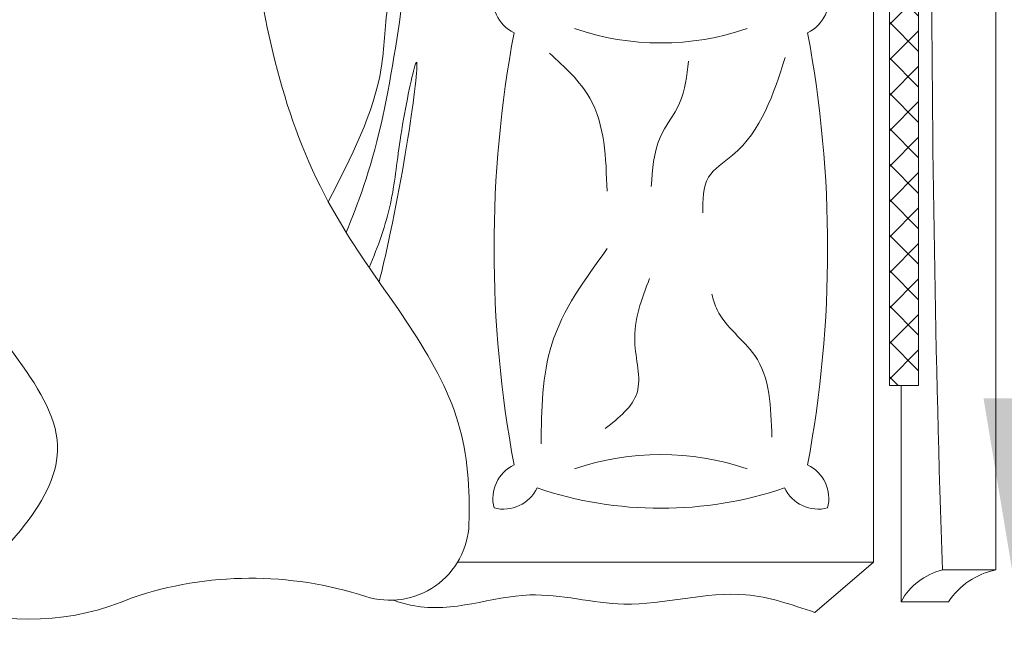
# Model space of a CAD drawing. Units: inches. Extents: x 2083 to 3317, y 1141 to 2115.
# Tile 239 of 256: x 3068 to 3114, y 1299 to 1327. Entities that reach past the tile are written whole.
import ezdxf

# ---------------------------------------------------------------- set-up
doc = ezdxf.new("R2010")
doc.units = ezdxf.units.IN
for name, color, linetype, lineweight in [('A-ANNO-DIMS', 2, 'Continuous', 18), ('A-FURN', 8, 'Continuous', 18), ('www.cadblocksfree.com', 7, 'Continuous', 9)]:
    doc.layers.add(name, color=color, linetype=linetype, lineweight=lineweight)
doc.layers.add('A-WALL-PATT', color=251, linetype='Continuous', lineweight=13, true_color=0x636466)
doc.styles.get("Standard").update_dxf_attribs({"font": 'arial.ttf'})
doc.dimstyles.new('ISO-25', dxfattribs={"dimtxt": 12, "dimasz": 12, "dimexe": 1.25, "dimexo": 0.625, "dimtad": 1, "dimlunit": 3, "dimtxsty": 'Standard', "dimcen": 2.5, "dimadec": 0, "dimazin": 0, "dimtfac": 1, "dimtmove": 0, "dimatfit": 3, "dimfxl": 1, "dimarcsym": 0})

# ---------------------------------------------------------------- blocks, each defined once
blk = doc.blocks.new('bed')
at = {"layer": 'www.cadblocksfree.com', "ltscale": 0.2}
h = blk.add_hatch(dxfattribs=at)
h.set_pattern_fill('ANSI37,_O', color=256, scale=0.393701)
h.set_pattern_definition([(45, (2420.7222, -262.9689), (-0.8838835, 0.8838835), []), (135, (2420.7222, -262.9689), (-0.8838835, -0.8838835), [])])
h.paths.add_polyline_path([(3417.573, 1472.402), (3372.192, 1472.402), (3372.192, 1470.941), (3417.573, 1470.941)])
for p, q in [((3426.763, 1473.586), (3426.763, 1476.249)), ((3372.192, 1472.402), (3417.573, 1472.402)), ((3417.573, 1470.941), (3417.573, 1472.402)), ((3372.192, 1470.941), (3417.573, 1470.941)), ((3426.379, 1470.154), (3428.883, 1467.22)), ((3409.943, 1443.853), (3408.408, 1442.961))]:
    blk.add_line(p, q, dxfattribs=at)
for points in [[(3426.763, 1476.249), (3363.002, 1476.249)], [(3417.573, 1471.524), (3428.347, 1471.524), (3428.347, 1473.886)], [(3426.379, 1449.413), (3426.379, 1470.154), (3363.387, 1470.154), (3363.387, 1447.076)]]:
    blk.add_lwpolyline(points, dxfattribs=at)
for centre, radius, start, end in [((3430.432, 1476.997), 3.744, 191.5225, 236.1729), ((3394.883, 2431.358), 958.303, 268.093559, 271.906441), ((3429.921, 1474.373), 3.255, 194.0061, 241.0824), ((3398.298, 1466.054), 1.87, 25.7901, 104.4834), ((3410.752, 1409.187), 58.677, 79.42346, 100.57654), ((3423.206, 1466.054), 1.87, 75.5166, 154.2099), ((3421.863, 1467.396), 1.87, 295.7901, 14.4834), ((3404.477, 1459.547), 19.215, 341.2852, 18.7148), ((3387.154, 1459.547), 13.338, 341.1598, 18.8402), ((3434.35, 1459.547), 13.338, 161.1598, 198.8402), ((3421.863, 1451.698), 1.87, 345.5166, 64.2099), ((3398.298, 1453.041), 1.87, 255.5166, 334.2099), ((3410.752, 1509.907), 58.677, 259.42346, 280.57654), ((3423.206, 1453.041), 1.87, 205.7901, 284.4834), ((3424.339, 1446.045), 3.937, 342.0511, 87.9851), ((3445.776, 1439.101), 18.596, 162.0511, 198.5657), ((3416.575, 1428.082), 12.646, 341.0268, 23.7782)]:
    blk.add_arc(centre, radius, start, end, dxfattribs=at)
for points, knots in [([(3428.883, 1467.22), (3428.494, 1466.08), (3427.438, 1462.983), (3429.036, 1458.154), (3427.377, 1452.621), (3429.083, 1448.872), (3428.374, 1446.522), (3428.273, 1446.192)], [0, 0, 0, 0, 0.0901802, 0.2449351, 0.3646438, 0.5132331, 0.5378548, 0.5378548, 0.5378548, 0.5378548]), ([(3401.221, 1465.744), (3403.047, 1465.161), (3405.408, 1464.407), (3407.088, 1461.635), (3408.312, 1461.638), (3408.953, 1461.64)], [0, 0, 0, 0, 5.530688, 7.154877, 8.940839, 8.940839, 8.940839, 8.940839]), ([(3420.141, 1465.083), (3418.661, 1465.041), (3416.141, 1464.969), (3414.502, 1462.52), (3413.283, 1462.165), (3413.011, 1462.086)], [0, 0, 0, 0, 4.163459, 7.093919, 7.934624, 7.934624, 7.934624, 7.934624]), ([(3401.408, 1460.927), (3402.126, 1460.846), (3403.512, 1460.689), (3405.283, 1459.224), (3406.806, 1459.127), (3407.654, 1459.073)], [0, 0, 0, 0, 2.127543, 4.10272, 6.58647, 6.58647, 6.58647, 6.58647]), ([(3419.716, 1456.774), (3419.174, 1457.459), (3418.052, 1458.876), (3415.084, 1457.893), (3413.26, 1458.594), (3412.241, 1458.985)], [0, 0, 0, 0, 2.388143, 4.935423, 8.166198, 8.166198, 8.166198, 8.166198]), ([(3400.996, 1453.995), (3401.698, 1454.761), (3403.498, 1456.726), (3406.222, 1456.811), (3407.884, 1456.863)], [0, 0, 0, 0, 3.013696, 7.735839, 7.735839, 7.735839, 7.735839]), ([(3420.479, 1453.579), (3418.77, 1453.599), (3415.179, 1453.639), (3412.269, 1455.762), (3410.745, 1456.874)], [0, 0, 0, 0, 5.002087, 10.507046, 10.507046, 10.507046, 10.507046]), ([(3409.943, 1443.853), (3413.12, 1445.837), (3417.433, 1449.66), (3422.724, 1450.042), (3424.477, 1449.98)], [1.3582378, 1.3582378, 1.3582378, 1.3582378, 1.6381418, 1.7706953, 1.7706953, 1.7706953, 1.7706953]), ([(3412.402, 1445.499), (3411.605, 1445.698), (3406.242, 1446.932), (3398.173, 1447.93), (3405.397, 1446.464), (3408.571, 1446.191), (3410.626, 1445.456), (3411.681, 1445)], [0.1043639, 0.1043639, 0.1043639, 0.1043639, 0.1489731, 0.3882761, 0.4793617, 0.5593494, 0.6446217, 0.6446217, 0.6446217, 0.6446217]), ([(3409.943, 1443.853), (3408.469, 1444.451), (3404.443, 1446.042), (3391.397, 1447.599), (3398.64, 1445.767), (3402.973, 1445.759), (3406.219, 1444.095), (3408.408, 1442.961)], [0.0056315, 0.0056315, 0.0056315, 0.0056315, 0.1489731, 0.3882761, 0.4793617, 0.5593494, 0.7397317, 0.7397317, 0.7397317, 0.7397317]), ([(3362.928, 1430.813), (3365.944, 1432.958), (3375.455, 1438.993), (3392.12, 1438.03), (3404.249, 1440.73), (3408.408, 1442.961)], [0.102872, 0.102872, 0.102872, 0.102872, 0.37972, 0.957702, 1.313793, 1.313793, 1.313793, 1.313793]), ([(3365.512, 1424.213), (3370.519, 1427.004), (3381.149, 1429.825), (3396.214, 1425.866), (3410.541, 1420.654), (3420.273, 1432.695), (3425.882, 1426.771), (3428.534, 1423.97)], [0.099185, 0.099185, 0.099185, 0.099185, 0.523647, 0.927087, 1.289918, 1.564439, 1.810555, 1.810555, 1.810555, 1.810555])]:
    blk.add_open_spline(points, degree=3, knots=knots, dxfattribs=at)
blk = doc.blocks.new('*D26')
at = {"layer": 'A-ANNO-DIMS', "color": 0, "lineweight": -2, "transparency": 16777216}
for p, q in [((3088.986, 1274.915), (3088.986, 1270.952)), ((3111.24, 1274.915), (3111.24, 1270.952)), ((3076.986, 1272.202), (2840.262, 1272.202)), ((3111.24, 1272.202), (3088.986, 1272.202)), ((3123.24, 1272.202), (3135.24, 1272.202))]:
    blk.add_line(p, q, dxfattribs=at)
at = {"layer": 'A-ANNO-DIMS', "color": 0, "transparency": 16777216}
for points in [[(3076.986, 1274.202), (3076.986, 1270.202), (3088.986, 1272.202)], [(3123.24, 1274.202), (3123.24, 1270.202), (3111.24, 1272.202)]]:
    blk.add_solid(points, dxfattribs=at)
at = {"layer": 'Defpoints', "color": 0, "transparency": 16777216}
for p in [(3088.986, 1275.54), (3111.24, 1275.54), (3088.986, 1272.202)]:
    blk.add_point(p, dxfattribs=at)
at = {"layer": 'A-ANNO-DIMS', "color": 0, "transparency": 16777216, "insert": (2952.624, 1279.032), "char_height": 12, "attachment_point": 5}
blk.add_mtext('NIGHTSTAND 1\'-10 1/2" TYP.', dxfattribs=at)
blk = doc.blocks.new('*D27')
at = {"layer": 'A-ANNO-DIMS', "color": 0, "lineweight": -2, "transparency": 16777216}
for p, q in [((3114.578, 1309.794), (3114.578, 1321.794)), ((3111.865, 1297.794), (3115.828, 1297.794)), ((3114.578, 1297.794), (3114.578, 1275.54)), ((3111.865, 1275.54), (3115.828, 1275.54)), ((3114.578, 1263.54), (3114.578, 1140.989))]:
    blk.add_line(p, q, dxfattribs=at)
at = {"layer": 'A-ANNO-DIMS', "color": 0, "transparency": 16777216}
for points in [[(3112.578, 1309.794), (3116.578, 1309.794), (3114.578, 1297.794)], [(3112.578, 1263.54), (3116.578, 1263.54), (3114.578, 1275.54)]]:
    blk.add_solid(points, dxfattribs=at)
at = {"layer": 'Defpoints', "color": 0, "transparency": 16777216}
for p in [(3111.24, 1297.794), (3111.24, 1275.54), (3114.578, 1275.54)]:
    blk.add_point(p, dxfattribs=at)
at = {"layer": 'A-ANNO-DIMS', "color": 0, "transparency": 16777216, "insert": (3107.749, 1196.264), "char_height": 12, "attachment_point": 5, "rotation": 90}
blk.add_mtext('1\'-10 1/2" TYP.', dxfattribs=at)

msp = doc.modelspace()

# ---------------------------------------------------------------- hatches: boundary and pattern name
at = {"layer": 'A-WALL-PATT'}
h = msp.add_hatch(color=256, dxfattribs=at)
h.dxf.hatch_style = 1
h.paths.add_polyline_path([(3126.96, 2020.761), (2748.96, 2020.761), (2604.96, 2020.761), (2226.96, 2020.761), (2226.96, 1702.761), (2466.96, 1702.761), (2466.96, 1582.761), (2418.96, 1582.761), (2418.96, 1477.761), (2226.96, 1477.761), (2226.96, 1263.261), (2544.96, 1263.261), (2544.96, 1411.761), (2604.96, 1411.761), (2685.96, 1411.761), (2685.96, 1420.761), (2604.96, 1420.761), (2604.96, 1573.761), (2604.96, 1702.761), (2604.96, 2011.761), (2748.96, 2011.761), (2748.96, 1702.761), (2862.96, 1702.761), (2862.96, 1621.761), (2871.96, 1621.761), (2871.96, 1702.761), (2883.96, 1702.761), (2883.96, 1706.939, -0.026459), (2883.96, 1711.761), (2757.96, 1711.761), (2757.96, 1807.761), (2787.96, 1807.761), (2787.96, 1812.261), (2757.96, 1812.261), (2757.96, 2011.761), (2877.96, 2011.761), (2877.96, 1812.261), (2847.96, 1812.261), (2847.96, 1807.761), (2889.836, 1807.761), (2889.836, 1812.261), (2882.46, 1812.261), (2882.46, 2011.761), (3117.96, 2011.761), (3117.96, 1812.261), (2937.836, 1812.261), (2937.836, 1807.761), (2995.71, 1807.761), (2995.71, 1796.118), (3000.21, 1796.118), (3000.21, 1807.761), (3117.96, 1807.761), (3117.96, 1711.761), (3000.21, 1711.761), (3000.21, 1760.118), (2998.573, 1760.118, -0.020711), (2995.71, 1760.118), (2995.71, 1711.761), (2931.96, 1711.761), (2931.96, 1702.761), (3126.96, 1702.761)])
h.paths.add_polyline_path([(2471.46, 2011.761), (2471.46, 1810.011), (2462.717, 1810.011), (2462.717, 1805.511), (2505.96, 1805.511), (2505.96, 1810.011), (2475.96, 1810.011), (2475.96, 2011.761), (2595.96, 2011.761), (2595.96, 1810.011), (2565.96, 1810.011), (2565.96, 1805.511), (2595.96, 1805.511), (2595.96, 1711.761), (2235.96, 1711.761), (2235.96, 1805.511), (2353.71, 1805.511), (2353.71, 1796.054), (2358.21, 1796.054), (2358.21, 1805.511), (2414.717, 1805.511), (2414.717, 1810.011), (2235.96, 1810.011), (2235.96, 2011.761)], flags=16)
h.paths.add_polyline_path([(2270.205, 1994.61), (2270.205, 1970.61), (2246.205, 1970.61), (2246.205, 1994.61)], flags=0)
edge = h.paths.add_edge_path(flags=0)
edge.add_ellipse((2332.027, 1899.798), major_axis=(-3.043, 3.043), ratio=0.168252, start_angle=-161.3322, end_angle=-156.3071, ccw=False)
edge.add_ellipse((2333.082, 1898.744), major_axis=(-1.055, 1.055), ratio=0.453532, start_angle=-123.371, end_angle=-94.1591)
edge = h.paths.add_edge_path(flags=0)
edge.add_ellipse((2332.027, 1968.876), major_axis=(3.043, 3.043), ratio=0.168252, start_angle=18.6678, end_angle=23.6929)
edge.add_spline(control_points=[(2332.926, 1970.691), (2332.227, 1970.336), (2330.894, 1969.659), (2328.413, 1970.932), (2327.204, 1967.749), (2324.71, 1969.956), (2322.533, 1967.012), (2320.013, 1971.296), (2317.68, 1968.158), (2316.041, 1967.102), (2315.427, 1966.81)], knot_values=[0, 0, 0, 0, 2.267059, 4.324559, 6.685584, 8.878641, 11.121502, 14.300359, 17.755284, 19.732645, 19.732645, 19.732645, 19.732645], degree=3, periodic=0)
edge.add_ellipse((2332.027, 1968.876), major_axis=(3.043, 3.043), ratio=0.168252, start_angle=18.6678, end_angle=23.6929, ccw=False)
edge.add_ellipse((2333.082, 1969.931), major_axis=(1.055, 1.055), ratio=0.453532, start_angle=56.629, end_angle=85.8409, ccw=False)
edge = h.paths.add_edge_path(flags=0)
edge.add_spline(control_points=[(2296.428, 1967.988), (2293.628, 1965.336), (2287.704, 1959.727), (2299.744, 1949.996), (2294.533, 1935.669), (2290.573, 1920.604), (2293.394, 1909.974), (2296.185, 1904.967)], knot_values=[0.099185, 0.099185, 0.099185, 0.099185, 0.345301, 0.619822, 0.982653, 1.386093, 1.810555, 1.810555, 1.810555, 1.810555], degree=3, periodic=0)
edge.add_spline(control_points=[(2296.185, 1904.967), (2297.384, 1902.619), (2298.001, 1901.949), (2298.553, 1901.468)], knot_values=[0.006246, 0.006246, 0.006246, 0.006246, 0.055476, 0.055476, 0.055476, 0.055476], degree=3, periodic=0)
edge.add_spline(control_points=[(2298.553, 1901.468), (2297.259, 1900.923), (2295.225, 1900.232), (2293.06, 1900.614), (2292.101, 1900.788), (2292.09, 1900.791)], knot_values=[0.312835, 0.312835, 0.312835, 0.312835, 0.40178, 0.474987, 0.475903, 0.475903, 0.475903, 0.475903], degree=3, periodic=0)
edge.add_arc((2292.794, 1904.664), 3.937, 215.4209, 259.6982, ccw=False)
edge.add_spline(control_points=[(2289.585, 1902.382), (2289.477, 1902.535), (2289.368, 1902.688), (2289.261, 1902.841)], knot_values=[0.102872, 0.102872, 0.102872, 0.102872, 0.116896, 0.116896, 0.116896, 0.116896], degree=3, periodic=0)
edge.add_spline(control_points=[(2289.261, 1902.841), (2288.687, 1902.55), (2287.64, 1902.02), (2285.881, 1901.874), (2283.853, 1901.504), (2281.72, 1899.711), (2278.467, 1899.493), (2276.157, 1901.883), (2272.259, 1899.804), (2267.778, 1901.843), (2262.244, 1900.184), (2257.415, 1901.782), (2254.318, 1900.726), (2253.178, 1900.337)], knot_values=[0, 0, 0, 0, 1.907977, 3.477176, 5.261074, 7.972851, 11.680248, 13.717921, 16.939592, 22.789562, 27.502503, 33.595215, 37.145618, 37.145618, 37.145618, 37.145618], degree=3, periodic=0)
edge.add_line((2253.178, 1900.337), (2250.244, 1902.841))
edge.add_line((2250.244, 1902.841), (2250.244, 1965.833))
edge.add_line((2250.244, 1965.833), (2253.178, 1968.337))
edge.add_spline(control_points=[(2253.178, 1968.337), (2254.318, 1967.948), (2257.415, 1966.892), (2262.244, 1968.49), (2267.778, 1966.831), (2271.527, 1968.537), (2273.876, 1967.828), (2274.207, 1967.728)], knot_values=[0, 0, 0, 0, 0.09018, 0.244935, 0.364644, 0.513233, 0.537855, 0.537855, 0.537855, 0.537855], degree=3, periodic=0)
edge.add_arc((2274.353, 1963.793), 3.937, 72.0511, 92.1279, ccw=False)
edge.add_arc((2281.297, 1985.23), 18.596, 252.0511, 288.5657)
edge.add_arc((2292.317, 1956.029), 12.646, 71.0268, 113.7782, ccw=False)
edge = h.paths.add_edge_path(flags=0)
edge.add_spline(control_points=[(2274.899, 1951.856), (2275.066, 1951.617), (2275.233, 1951.377), (2275.398, 1951.136)], knot_values=[1.409916, 1.409916, 1.409916, 1.409916, 1.43159, 1.43159, 1.43159, 1.43159], degree=3, periodic=0)
edge.add_spline(control_points=[(2275.398, 1951.136), (2275.792, 1950.562), (2276.179, 1949.984), (2276.546, 1949.397)], knot_values=[1.358238, 1.358238, 1.358238, 1.358238, 1.409916, 1.409916, 1.409916, 1.409916], degree=3, periodic=0)
edge.add_line((2276.546, 1949.397), (2277.437, 1947.862))
edge.add_spline(control_points=[(2277.437, 1947.862), (2276.304, 1945.673), (2274.64, 1942.427), (2274.632, 1938.094), (2272.799, 1930.852), (2274.356, 1943.897), (2275.948, 1947.923), (2276.546, 1949.397)], knot_values=[0.005632, 0.005632, 0.005632, 0.005632, 0.186014, 0.266002, 0.357087, 0.59639, 0.739732, 0.739732, 0.739732, 0.739732], degree=3, periodic=0)
edge.add_spline(control_points=[(2276.546, 1949.397), (2276.179, 1949.984), (2275.792, 1950.562), (2275.398, 1951.136)], knot_values=[1.358238, 1.358238, 1.358238, 1.358238, 1.409916, 1.409916, 1.409916, 1.409916], degree=3, periodic=0)
edge.add_spline(control_points=[(2275.398, 1951.136), (2274.943, 1950.08), (2274.208, 1948.025), (2273.935, 1944.851), (2272.469, 1937.627), (2273.466, 1945.696), (2274.701, 1951.059), (2274.899, 1951.856)], knot_values=[0.104364, 0.104364, 0.104364, 0.104364, 0.189636, 0.269624, 0.36071, 0.600013, 0.644622, 0.644622, 0.644622, 0.644622], degree=3, periodic=0)
h.paths.add_polyline_path([(2269.168, 1963.128, -0.357527), (2268.171, 1960.976, -0.092561), (2268.171, 1939.436, -0.357527), (2269.168, 1937.285, -0.357527), (2267.016, 1938.282, -0.164785), (2254.686, 1938.282, -0.357527), (2252.534, 1937.285, -0.357527), (2253.531, 1939.436, -0.092561), (2253.531, 1960.976, -0.357527), (2252.534, 1963.128, -0.357527), (2254.686, 1962.131, -0.164785), (2267.016, 1962.131, -0.357527)], flags=0)
h.paths.add_polyline_path([(2248.874, 1967.802), (2248.874, 1957.028), (2249.458, 1957.028), (2249.458, 1911.647), (2248.874, 1911.647), (2248.874, 1900.873), (2246.512, 1900.873, 0.197327), (2244.15, 1902.457), (2244.15, 1966.218, 0.197327), (2246.512, 1967.802)], flags=0)
h.paths.add_polyline_path([(2269.168, 1931.389, -0.357527), (2268.171, 1929.238, -0.092561), (2268.171, 1907.698, -0.357527), (2269.168, 1905.547, -0.357527), (2267.016, 1906.544, -0.164785), (2254.686, 1906.544, -0.357527), (2252.534, 1905.547, -0.357527), (2253.531, 1907.698, -0.092561), (2253.531, 1929.238, -0.357527), (2252.534, 1931.389, -0.357527), (2254.686, 1930.392, -0.164785), (2267.016, 1930.392, -0.357527)], flags=0)
edge = h.paths.add_edge_path(flags=0)
edge.add_spline(control_points=[(2276.197, 1906.724), (2276.168, 1909.029), (2276.114, 1913.372), (2270.598, 1924.925), (2273.905, 1919.013), (2275.922, 1916.262), (2275.475, 1912.402), (2277.258, 1910.381), (2276.696, 1908.225), (2276.646, 1906.813), (2276.618, 1906.008)], knot_values=[0, 0, 0, 0, 8.61026, 16.221274, 18.843057, 23.804898, 27.440828, 29.356102, 31.203478, 33.650687, 33.650687, 33.650687, 33.650687], degree=3, periodic=0)
edge.add_spline(control_points=[(2276.618, 1906.008), (2276.623, 1905.624), (2276.498, 1904.629), (2275.442, 1903.855), (2274.937, 1903.08), (2274.859, 1902.841)], knot_values=[0.156488, 0.156488, 0.156488, 0.156488, 0.184398, 0.231376, 0.250598, 0.250598, 0.250598, 0.250598], degree=3, periodic=0)
edge.add_line((2274.859, 1902.841), (2276.506, 1902.841))
edge.add_spline(control_points=[(2276.506, 1902.841), (2276.788, 1903.085), (2277.665, 1904.125), (2278.25, 1904.341), (2277.654, 1908.527), (2278.156, 1906.228), (2278.1, 1905.286), (2278.847, 1904.069), (2277.857, 1903.415), (2277.874, 1902.991), (2277.904, 1902.841)], knot_values=[0.059574, 0.059574, 0.059574, 0.059574, 0.080753, 0.103741, 0.16972, 0.176036, 0.207137, 0.240474, 0.262341, 0.27366, 0.27366, 0.27366, 0.27366], degree=3, periodic=0)
edge.add_line((2277.904, 1902.841), (2280.03, 1902.841))
edge.add_spline(control_points=[(2280.03, 1902.841), (2279.888, 1903.088), (2279.499, 1903.982), (2280.152, 1905.939), (2278.104, 1909.658), (2279.762, 1907.185), (2280.328, 1904.875), (2280.485, 1903.49), (2281.463, 1903.249), (2281.758, 1902.936), (2281.834, 1902.841)], knot_values=[0.013856, 0.013856, 0.013856, 0.013856, 0.034874, 0.088867, 0.107879, 0.126738, 0.158714, 0.193757, 0.217487, 0.226722, 0.226722, 0.226722, 0.226722], degree=3, periodic=0)
edge.add_spline(control_points=[(2281.834, 1902.841), (2281.788, 1902.827), (2281.647, 1902.783), (2281.396, 1902.859), (2281.088, 1902.985), (2280.721, 1903.061), (2280.333, 1903.026), (2280.125, 1902.899), (2280.03, 1902.841)], knot_values=[0, 0, 0, 0, 0.14413, 0.435517, 0.749276, 1.153046, 1.548371, 1.878348, 1.878348, 1.878348, 1.878348], degree=3, periodic=0)
edge.add_line((2280.03, 1902.841), (2277.904, 1902.841))
edge.add_spline(control_points=[(2277.904, 1902.841), (2277.893, 1902.796), (2277.865, 1902.68), (2277.607, 1902.687), (2277.274, 1902.801), (2276.838, 1902.62), (2276.584, 1902.789), (2276.506, 1902.841)], knot_values=[0, 0, 0, 0, 0.127189, 0.326199, 0.628009, 1.24357, 1.515331, 1.515331, 1.515331, 1.515331], degree=3, periodic=0)
edge.add_line((2276.506, 1902.841), (2274.859, 1902.841))
edge.add_spline(control_points=[(2274.859, 1902.841), (2274.814, 1902.899), (2274.725, 1903.013), (2274.493, 1903.119), (2274.244, 1902.961), (2273.937, 1903.185), (2273.614, 1902.983), (2273.408, 1902.883), (2273.322, 1902.841)], knot_values=[0, 0, 0, 0, 0.21843, 0.436957, 0.687977, 0.990379, 1.398396, 1.69185, 1.69185, 1.69185, 1.69185], degree=3, periodic=0)
edge.add_spline(control_points=[(2273.322, 1902.841), (2273.617, 1903.446), (2274.274, 1904.538), (2276.027, 1904.574), (2276.207, 1906.584), (2276.197, 1906.724)], knot_values=[0.012227, 0.012227, 0.012227, 0.012227, 0.059472, 0.106218, 0.134458, 0.134458, 0.134458, 0.134458], degree=3, periodic=0)
h.paths.add_polyline_path([(2270.776, 1897.79), (2270.776, 1873.79), (2246.776, 1873.79), (2246.776, 1897.79)], flags=0)
h.paths.add_polyline_path([(2353.71, 1760.005), (2353.71, 1760.054), (2358.21, 1760.054, -0.033729)], flags=0)
h.paths.add_polyline_path([(2321.819, 1737.529), (2341.995, 1737.529, -0.414214), (2343.203, 1736.321), (2343.203, 1721.021, -0.414214), (2341.995, 1719.813), (2321.819, 1719.813, -0.414214), (2320.611, 1721.021), (2320.611, 1736.321, -0.414214)], flags=0)
h.paths.add_polyline_path([(2324.235, 1736.321), (2339.579, 1736.321, -0.414214), (2341.995, 1733.905), (2341.995, 1725.45, -0.414214), (2339.579, 1723.034), (2333.681, 1723.034), (2333.845, 1722.045, -0.870646), (2335.425, 1721.826, -0.767327), (2333.923, 1721.423), (2331.291, 1721.423, -0.767327), (2329.788, 1721.826, -0.870646), (2331.368, 1722.045), (2331.533, 1723.034), (2324.235, 1723.034, -0.414214), (2321.819, 1725.45), (2321.819, 1733.905, -0.414214)], flags=0)
h.paths.add_polyline_path([(2570.484, 1928.615), (2589.684, 1928.615), (2590.169, 1928.615), (2590.169, 1904.993), (2570.484, 1904.993)], flags=0)
h.paths.add_polyline_path([(2574.447, 1927.264, -1), (2572.829, 1927.264, -1)], flags=0)
h.paths.add_polyline_path([(2573.09, 1926.941), (2573.925, 1927.776), (2574.148, 1927.553), (2573.313, 1926.718)], flags=0)
h.paths.add_polyline_path([(2578.779, 1919.73, -1), (2571.592, 1919.73, -1)], flags=0)
h.paths.add_polyline_path([(2578.385, 1919.73, -1), (2571.985, 1919.73, -1)], flags=0)
h.paths.add_polyline_path([(2331.596, 1729.476, -1), (2333.618, 1729.476, -1)], flags=0)
h.paths.add_polyline_path([(2578.034, 1927.264, -1), (2576.416, 1927.264, -1)], flags=0)
h.paths.add_polyline_path([(2576.689, 1927.531), (2576.912, 1927.754), (2577.747, 1926.919), (2577.524, 1926.696)], flags=0)
h.paths.add_polyline_path([(2578.139, 1909.86, -1), (2572.232, 1909.86, -1)], flags=0)
h.paths.add_polyline_path([(2577.745, 1909.86, -1), (2572.625, 1909.86, -1)], flags=0)
h.paths.add_polyline_path([(2583.798, 1927.264, -1), (2582.179, 1927.264, -1)], flags=0)
h.paths.add_polyline_path([(2582.719, 1927.754), (2583.554, 1926.919), (2583.331, 1926.696), (2582.496, 1927.531)], flags=0)
h.paths.add_polyline_path([(2582.496, 1927.531), (2582.719, 1927.754), (2583.554, 1926.919), (2583.331, 1926.696)], flags=0)
h.paths.add_polyline_path([(2587.739, 1920.53, -1), (2581.832, 1920.53, -1)], flags=0)
h.paths.add_polyline_path([(2587.345, 1920.53, -1), (2582.225, 1920.53, -1)], flags=0)
h.paths.add_polyline_path([(2587.385, 1927.264, -1), (2585.766, 1927.264, -1)], flags=0)
h.paths.add_polyline_path([(2586.082, 1926.98), (2586.917, 1927.815), (2587.14, 1927.593), (2586.305, 1926.758)], flags=0)
h.paths.add_polyline_path([(2588.379, 1910.66, -1), (2581.192, 1910.66, -1)], flags=0)
h.paths.add_polyline_path([(2587.985, 1910.66, -1), (2581.585, 1910.66, -1)], flags=0)
h.paths.add_polyline_path([(2417.168, 1729.478), (2437.344, 1729.478, -0.414214), (2438.552, 1728.27), (2438.552, 1712.969, -0.414214), (2437.344, 1711.761), (2417.168, 1711.761, -0.414214), (2415.96, 1712.969), (2415.96, 1728.27, -0.414214)], flags=0)
h.paths.add_polyline_path([(2419.584, 1728.27), (2434.928, 1728.27, -0.414214), (2437.344, 1725.854), (2437.344, 1717.398, -0.414214), (2434.928, 1714.983), (2429.029, 1714.983), (2429.194, 1713.994, -0.870646), (2430.774, 1713.775, -0.767327), (2429.271, 1713.372), (2426.64, 1713.372, -0.767327), (2425.137, 1713.775, -0.870646), (2426.717, 1713.994), (2426.882, 1714.983), (2419.584, 1714.983, -0.414214), (2417.168, 1717.398), (2417.168, 1725.854, -0.414214)], flags=0)
h.paths.add_polyline_path([(2419.584, 1728.27), (2434.928, 1728.27, -0.414214), (2437.344, 1725.854), (2437.344, 1717.398, -0.414214), (2434.928, 1714.983), (2429.029, 1714.983), (2428.358, 1719.009), (2427.553, 1719.009), (2426.882, 1714.983), (2419.584, 1714.983, -0.414214), (2417.168, 1717.398), (2417.168, 1725.854, -0.414214)], flags=0)
h.paths.add_polyline_path([(2426.944, 1721.425, -1), (2428.967, 1721.425, -1)], flags=0)
h.paths.add_polyline_path([(2475.96, 1702.761), (2595.96, 1702.761), (2595.96, 1582.761), (2475.96, 1582.761)], flags=16)
h.paths.add_polyline_path([(2427.96, 1573.761), (2595.96, 1573.761), (2595.96, 1468.761), (2595.96, 1420.761), (2384.46, 1420.761), (2384.46, 1468.761), (2427.96, 1468.761)], flags=16)
h.paths.add_polyline_path([(2379.96, 1468.761), (2379.96, 1420.761), (2235.96, 1420.761), (2235.96, 1468.761)], flags=16)
h.paths.add_polyline_path([(2317.816, 1466.696), (2337.992, 1466.696, -0.414214), (2339.2, 1465.488), (2339.2, 1450.187, -0.414214), (2337.992, 1448.979), (2317.816, 1448.979, -0.414214), (2316.608, 1450.187), (2316.608, 1465.488, -0.414214)], flags=0)
h.paths.add_polyline_path([(2320.232, 1465.488), (2335.576, 1465.488, -0.414214), (2337.992, 1463.072), (2337.992, 1454.616, -0.414214), (2335.576, 1452.2), (2329.677, 1452.2), (2329.842, 1451.212, -0.870646), (2331.422, 1450.992, -0.767327), (2329.92, 1450.59), (2327.288, 1450.59, -0.767327), (2325.785, 1450.992, -0.870646), (2327.365, 1451.212), (2327.53, 1452.2), (2320.232, 1452.2, -0.414214), (2317.816, 1454.616), (2317.816, 1463.072, -0.414214)], flags=0)
h.paths.add_polyline_path([(2320.232, 1465.488), (2335.576, 1465.488, -0.414214), (2337.992, 1463.072), (2337.992, 1454.616, -0.414214), (2335.576, 1452.2), (2329.677, 1452.2), (2329.006, 1456.227), (2328.201, 1456.227), (2327.53, 1452.2), (2320.232, 1452.2, -0.414214), (2317.816, 1454.616), (2317.816, 1463.072, -0.414214)], flags=0)
h.paths.add_polyline_path([(2327.593, 1458.643, -1), (2329.615, 1458.643, -1)], flags=0)
h.paths.add_polyline_path([(2244.412, 1433.34), (2241.921, 1433.34, -0.414214), (2240.018, 1435.244), (2240.018, 1440.953, -0.414211), (2241.921, 1442.856), (2244.412, 1442.856, -1.976472)], flags=0)
h.paths.add_polyline_path([(2245.357, 1434.398, -0.414214), (2245.357, 1441.799, -2.144098)], flags=0)
h.paths.add_polyline_path([(2535.96, 1416.261), (2535.96, 1272.261), (2235.96, 1272.261), (2235.96, 1416.261)], flags=16)
h.paths.add_polyline_path([(2260.12, 1384.293), (2260.12, 1362.039), (2237.865, 1362.039), (2237.865, 1384.293)], flags=0)
edge = h.paths.add_edge_path(flags=0)
edge.add_line((2318.252, 1362.093), (2318.146, 1362.001))
edge.add_ellipse((2317.445, 1360.431), major_axis=(2.822, 2.822), ratio=0.168252, start_angle=18.6678, end_angle=20.9481, ccw=False)
edge.add_ellipse((2318.423, 1361.409), major_axis=(0.978, 0.978), ratio=0.453532, start_angle=56.629, end_angle=70.2262, ccw=False)
edge = h.paths.add_edge_path(flags=0)
edge.add_line((2319.107, 1295.571), (2319.015, 1295.677))
edge.add_ellipse((2317.445, 1296.378), major_axis=(-2.822, 2.822), ratio=0.168252, start_angle=-161.3322, end_angle=-159.0519, ccw=False)
edge.add_ellipse((2318.423, 1295.4), major_axis=(-0.978, 0.978), ratio=0.453532, start_angle=-123.371, end_angle=-109.7738)
edge = h.paths.add_edge_path(flags=0)
edge.add_spline(control_points=[(2284.21, 1301.17), (2284.581, 1300.445), (2284.891, 1299.892), (2285.16, 1299.461)], knot_values=[0.039066, 0.039066, 0.039066, 0.039066, 0.055476, 0.055476, 0.055476, 0.055476], degree=3, periodic=0)
edge.add_line((2285.16, 1299.461), (2284.21, 1301.17))
edge = h.paths.add_edge_path(flags=0)
edge.add_line((2280.412, 1297.298), (2283.37, 1297.036))
edge.add_line((2283.37, 1297.036), (2286.406, 1297.926))
edge.add_spline(control_points=[(2286.406, 1297.926), (2285.305, 1297.463), (2284.345, 1297.129), (2283.37, 1297.036)], knot_values=[0.394369, 0.394369, 0.394369, 0.394369, 0.475903, 0.475903, 0.475903, 0.475903], degree=3, periodic=0)
edge.add_spline(control_points=[(2283.37, 1297.036), (2283.281, 1297.028), (2282.316, 1296.957), (2281.313, 1297.134), (2280.423, 1297.296), (2280.412, 1297.298)], knot_values=[0.312835, 0.312835, 0.312835, 0.312835, 0.320246, 0.393453, 0.394369, 0.394369, 0.394369, 0.394369], degree=3, periodic=0)
edge = h.paths.add_edge_path(flags=0)
edge.add_line((2284.436, 1359.607), (2280.446, 1355.328))
edge.add_line((2280.446, 1355.328), (2279.58, 1351.018))
edge.add_line((2279.58, 1351.018), (2282.413, 1346.58))
edge.add_spline(control_points=[(2282.413, 1346.58), (2283.153, 1345.589), (2284.253, 1344.029), (2284.801, 1342.387), (2284.935, 1341.806)], knot_values=[1.240098, 1.240098, 1.240098, 1.240098, 1.332892, 1.382712, 1.382712, 1.382712, 1.382712], degree=3, periodic=0)
edge.add_spline(control_points=[(2284.935, 1341.806), (2285.319, 1340.141), (2285.233, 1338.409), (2284.91, 1336.654)], knot_values=[1.097484, 1.097484, 1.097484, 1.097484, 1.240098, 1.240098, 1.240098, 1.240098], degree=3, periodic=0)
edge.add_spline(control_points=[(2284.91, 1336.654), (2284.587, 1334.899), (2284.027, 1333.12), (2283.463, 1331.361)], knot_values=[0.95487, 0.95487, 0.95487, 0.95487, 1.097484, 1.097484, 1.097484, 1.097484], degree=3, periodic=0)
edge.add_line((2283.463, 1331.361), (2281.89, 1326.153))
edge.add_line((2281.89, 1326.153), (2280.756, 1321.056))
edge.add_line((2280.756, 1321.056), (2280.299, 1316.002))
edge.add_line((2280.299, 1316.002), (2280.716, 1310.95))
edge.add_line((2280.716, 1310.95), (2282.028, 1305.972))
edge.add_line((2282.028, 1305.972), (2284.21, 1301.17))
edge.add_spline(control_points=[(2284.21, 1301.17), (2283.341, 1302.73), (2282.612, 1304.336), (2282.028, 1305.972)], knot_values=[0.099185, 0.099185, 0.099185, 0.099185, 0.241799, 0.241799, 0.241799, 0.241799], degree=3, periodic=0)
edge.add_spline(control_points=[(2282.028, 1305.972), (2281.444, 1307.608), (2281.005, 1309.273), (2280.716, 1310.95)], knot_values=[0.241799, 0.241799, 0.241799, 0.241799, 0.384413, 0.384413, 0.384413, 0.384413], degree=3, periodic=0)
edge.add_spline(control_points=[(2280.716, 1310.95), (2280.433, 1312.588), (2280.289, 1314.277), (2280.299, 1315.962), (2280.299, 1316.002)], knot_values=[0.384413, 0.384413, 0.384413, 0.384413, 0.523647, 0.527028, 0.527028, 0.527028, 0.527028], degree=3, periodic=0)
edge.add_spline(control_points=[(2280.299, 1316.002), (2280.312, 1317.687), (2280.478, 1319.368), (2280.756, 1321.056)], knot_values=[0.527028, 0.527028, 0.527028, 0.527028, 0.669642, 0.669642, 0.669642, 0.669642], degree=3, periodic=0)
edge.add_spline(control_points=[(2280.756, 1321.056), (2281.035, 1322.744), (2281.426, 1324.44), (2281.89, 1326.153)], knot_values=[0.669642, 0.669642, 0.669642, 0.669642, 0.812256, 0.812256, 0.812256, 0.812256], degree=3, periodic=0)
edge.add_spline(control_points=[(2281.89, 1326.153), (2282.264, 1327.533), (2282.788, 1329.262), (2283.353, 1331.018), (2283.463, 1331.361)], knot_values=[0.812256, 0.812256, 0.812256, 0.812256, 0.927087, 0.95487, 0.95487, 0.95487, 0.95487], degree=3, periodic=0)
edge.add_line((2283.463, 1331.361), (2284.91, 1336.654))
edge.add_line((2284.91, 1336.654), (2284.935, 1341.806))
edge.add_line((2284.935, 1341.806), (2282.413, 1346.58))
edge.add_spline(control_points=[(2282.413, 1346.58), (2281.275, 1348.104), (2280.078, 1349.57), (2279.58, 1351.018)], knot_values=[1.382712, 1.382712, 1.382712, 1.382712, 1.525326, 1.525326, 1.525326, 1.525326], degree=3, periodic=0)
edge.add_spline(control_points=[(2279.58, 1351.018), (2279.443, 1351.415), (2279.136, 1352.857), (2279.735, 1354.29), (2280.446, 1355.328)], knot_values=[1.525326, 1.525326, 1.525326, 1.525326, 1.564439, 1.667941, 1.667941, 1.667941, 1.667941], degree=3, periodic=0)
edge.add_spline(control_points=[(2280.446, 1355.328), (2281.426, 1356.758), (2282.931, 1358.183), (2284.436, 1359.607)], knot_values=[1.667941, 1.667941, 1.667941, 1.667941, 1.810555, 1.810555, 1.810555, 1.810555], degree=3, periodic=0)
edge.add_arc((2280.623, 1348.518), 11.726, 71.0268, 113.7782)
edge.add_arc((2270.405, 1375.595), 17.244, 252.0511, 288.5657, ccw=False)
edge.add_arc((2263.966, 1355.718), 3.651, 72.0511, 92.1279)
edge.add_arc((2263.966, 1355.718), 3.651, 92.1279, 177.9851)
edge.add_spline(control_points=[(2260.318, 1355.846), (2260.26, 1354.221), (2260.551, 1350.187), (2262.999, 1346.766), (2264.473, 1344.649)], knot_values=[1.43159, 1.43159, 1.43159, 1.43159, 1.564144, 1.770695, 1.770695, 1.770695, 1.770695], degree=3, periodic=0)
edge.add_line((2264.473, 1344.649), (2264.936, 1343.983))
edge.add_spline(control_points=[(2263.801, 1340.248), (2263.843, 1340.514), (2264.067, 1341.756), (2264.513, 1343.002), (2264.935, 1343.981)], knot_values=[0.53657, 0.53657, 0.53657, 0.53657, 0.559349, 0.644622, 0.644622, 0.644622, 0.644622], degree=3, periodic=0)
edge.add_spline(control_points=[(2264.935, 1343.981), (2265.118, 1343.715), (2265.299, 1343.448), (2265.477, 1343.179)], knot_values=[1.384077, 1.384077, 1.384077, 1.384077, 1.409916, 1.409916, 1.409916, 1.409916], degree=3, periodic=0)
edge.add_spline(control_points=[(2265.477, 1343.179), (2265.655, 1342.911), (2265.829, 1342.641), (2265.999, 1342.369)], knot_values=[1.358238, 1.358238, 1.358238, 1.358238, 1.384077, 1.384077, 1.384077, 1.384077], degree=3, periodic=0)
edge.add_line((2265.999, 1342.369), (2266.826, 1340.946))
edge.add_spline(control_points=[(2266.826, 1340.946), (2268.894, 1337.09), (2271.398, 1325.843), (2270.516, 1310.569), (2275.919, 1301.861), (2277.79, 1299.199)], knot_values=[0.116896, 0.116896, 0.116896, 0.116896, 0.472987, 1.050969, 1.313793, 1.313793, 1.313793, 1.313793], degree=3, periodic=0)
edge.add_spline(control_points=[(2277.79, 1299.199), (2277.839, 1299.128), (2277.889, 1299.057), (2277.94, 1298.987)], knot_values=[0.109884, 0.109884, 0.109884, 0.109884, 0.116896, 0.116896, 0.116896, 0.116896], degree=3, periodic=0)
edge.add_line((2277.94, 1298.987), (2277.789, 1299.199))
edge.add_spline(control_points=[(2277.789, 1299.199), (2277.257, 1298.929), (2276.286, 1298.438), (2275.039, 1298.334), (2274.383, 1298.239), (2274.215, 1298.209)], knot_values=[33.12187, 33.12187, 33.12187, 33.12187, 35.029056, 36.598255, 37.144827, 37.144827, 37.144827, 37.144827], degree=3, periodic=0)
edge.add_line((2274.215, 1298.209), (2273.073, 1297.893))
edge.add_spline(control_points=[(2273.073, 1297.893), (2272.323, 1297.58), (2271.039, 1296.511), (2269.248, 1296.226), (2268.423, 1296.375)], knot_values=[26.532584, 26.532584, 26.532584, 26.532584, 29.198919, 31.839101, 31.839101, 31.839101, 31.839101], degree=3, periodic=0)
edge.add_line((2268.423, 1296.375), (2263.879, 1297.458))
edge.add_spline(control_points=[(2263.879, 1297.458), (2263.556, 1297.359), (2261.86, 1296.839), (2260.239, 1297.282), (2258.933, 1297.516)], knot_values=[15.919551, 15.919551, 15.919551, 15.919551, 16.939592, 21.226067, 21.226067, 21.226067, 21.226067], degree=3, periodic=0)
edge.add_line((2258.933, 1297.516), (2254.055, 1297.329))
edge.add_spline(control_points=[(2254.055, 1297.329), (2253.756, 1297.296), (2252.114, 1297.165), (2250.462, 1297.544), (2249.13, 1297.668)], knot_values=[5.306517, 5.306517, 5.306517, 5.306517, 6.276435, 10.613034, 10.613034, 10.613034, 10.613034], degree=3, periodic=0)
edge.add_line((2249.13, 1297.668), (2244.332, 1296.878))
edge.add_line((2244.332, 1296.878), (2241.611, 1299.199))
edge.add_line((2241.611, 1299.199), (2241.611, 1357.609))
edge.add_line((2241.611, 1357.609), (2244.332, 1359.931))
edge.add_line((2244.332, 1359.931), (2252.729, 1359.543))
edge.add_spline(control_points=[(2252.729, 1359.543), (2252.871, 1359.546), (2253.306, 1359.548), (2253.74, 1359.514), (2254.032, 1359.482)], knot_values=[0.233291, 0.233291, 0.233291, 0.233291, 0.244935, 0.268927, 0.268927, 0.268927, 0.268927], degree=3, periodic=0)
edge.add_line((2254.032, 1359.482), (2259.587, 1359.416))
edge.add_spline(control_points=[(2259.587, 1359.416), (2260.677, 1359.629), (2262.073, 1359.897), (2263.524, 1359.459), (2263.83, 1359.366)], knot_values=[0.422516, 0.422516, 0.422516, 0.422516, 0.513233, 0.537855, 0.537855, 0.537855, 0.537855], degree=3, periodic=0)
edge.add_arc((2263.966, 1355.718), 3.651, 72.0511, 92.1279, ccw=False)
edge.add_arc((2270.405, 1375.595), 17.244, 252.0511, 288.5657)
edge.add_arc((2280.623, 1348.518), 11.726, 71.0268, 113.7782, ccw=False)
h.paths.add_polyline_path([(2240.341, 1359.435), (2240.341, 1349.444), (2240.882, 1349.444), (2240.882, 1307.365), (2240.341, 1307.365), (2240.341, 1297.374), (2238.15, 1297.374, 0.197327), (2235.96, 1298.843), (2235.96, 1357.966, 0.197327), (2238.15, 1359.435)], flags=0)
h.paths.add_polyline_path([(2259.158, 1355.101, -0.357527), (2258.233, 1353.106, -0.092561), (2258.233, 1333.133, -0.357527), (2259.158, 1331.138, -0.357527), (2257.163, 1332.062, -0.164785), (2245.729, 1332.062, -0.357527), (2243.735, 1331.138, -0.357527), (2244.659, 1333.133, -0.092561), (2244.659, 1353.106, -0.357527), (2243.735, 1355.101, -0.357527), (2245.729, 1354.176, -0.164785), (2257.163, 1354.176, -0.357527)], flags=0)
edge = h.paths.add_edge_path(flags=0)
edge.add_line((2265.999, 1342.369), (2266.826, 1340.946))
edge.add_line((2266.826, 1340.946), (2265.308, 1337.814))
edge.add_line((2265.308, 1337.814), (2264.358, 1334.653))
edge.add_line((2264.358, 1334.653), (2264.262, 1333.8))
edge.add_spline(control_points=[(2264.262, 1333.8), (2264.208, 1333.187), (2264.162, 1332.366), (2264.007, 1331.414), (2263.969, 1331.202)], knot_values=[0.464444, 0.464444, 0.464444, 0.464444, 0.516691, 0.531608, 0.531608, 0.531608, 0.531608], degree=3, periodic=0)
edge.add_spline(control_points=[(2263.969, 1331.202), (2263.775, 1330.119), (2263.424, 1328.791), (2263.257, 1328.531), (2263.234, 1328.515)], knot_values=[0.372682, 0.372682, 0.372682, 0.372682, 0.44885, 0.464444, 0.464444, 0.464444, 0.464444], degree=3, periodic=0)
edge.add_spline(control_points=[(2263.234, 1328.515), (2263.096, 1328.42), (2263.131, 1329.301), (2263.275, 1330.616)], knot_values=[0.280919, 0.280919, 0.280919, 0.280919, 0.372682, 0.372682, 0.372682, 0.372682], degree=3, periodic=0)
edge.add_spline(control_points=[(2263.275, 1330.616), (2263.419, 1331.93), (2263.672, 1333.677), (2263.97, 1335.315)], knot_values=[0.189157, 0.189157, 0.189157, 0.189157, 0.280919, 0.280919, 0.280919, 0.280919], degree=3, periodic=0)
edge.add_spline(control_points=[(2263.97, 1335.315), (2264.1, 1336.032), (2264.419, 1337.622), (2264.755, 1338.864), (2264.947, 1339.491)], knot_values=[0.097394, 0.097394, 0.097394, 0.097394, 0.137578, 0.189157, 0.189157, 0.189157, 0.189157], degree=3, periodic=0)
edge.add_spline(control_points=[(2264.947, 1339.491), (2265.29, 1340.606), (2265.644, 1341.494), (2265.999, 1342.369)], knot_values=[0.005632, 0.005632, 0.005632, 0.005632, 0.097394, 0.097394, 0.097394, 0.097394], degree=3, periodic=0)
h.paths.add_polyline_path([(2259.158, 1325.671, -0.357527), (2258.233, 1323.676, -0.092561), (2258.233, 1303.703, -0.357527), (2259.158, 1301.708, -0.357527), (2257.163, 1302.633, -0.164785), (2245.729, 1302.633, -0.357527), (2243.735, 1301.708, -0.357527), (2244.659, 1303.703, -0.092561), (2244.659, 1323.676, -0.357527), (2243.735, 1325.671, -0.357527), (2245.729, 1324.747, -0.164785), (2257.163, 1324.747, -0.357527)], flags=0)
edge = h.paths.add_edge_path(flags=0)
edge.add_spline(control_points=[(2261.709, 1317.311), (2261.679, 1317.418), (2261.762, 1317.389), (2262.491, 1316.09), (2262.962, 1315.301)], knot_values=[14.955861, 14.955861, 14.955861, 14.955861, 16.221274, 18.694826, 18.694826, 18.694826, 18.694826], degree=3, periodic=0)
edge.add_spline(control_points=[(2262.962, 1315.301), (2262.99, 1315.254), (2263.702, 1314.067), (2264.349, 1313.127), (2264.73, 1312.164)], knot_values=[18.694826, 18.694826, 18.694826, 18.694826, 18.843057, 22.433791, 22.433791, 22.433791, 22.433791], degree=3, periodic=0)
edge.add_spline(control_points=[(2264.73, 1312.164), (2264.876, 1311.796), (2265.177, 1310.77), (2265.143, 1309.559), (2265.248, 1308.824)], knot_values=[22.433791, 22.433791, 22.433791, 22.433791, 23.804898, 26.172756, 26.172756, 26.172756, 26.172756], degree=3, periodic=0)
edge.add_line((2265.248, 1308.824), (2265.851, 1307.172))
edge.add_spline(control_points=[(2265.851, 1307.172), (2266.065, 1306.822), (2266.384, 1306.332), (2266.424, 1305.781), (2266.42, 1305.611)], knot_values=[28.062562, 28.062562, 28.062562, 28.062562, 29.356102, 29.911721, 29.911721, 29.911721, 29.911721], degree=3, periodic=0)
edge.add_spline(control_points=[(2266.42, 1305.611), (2266.416, 1305.433), (2266.394, 1305.25), (2266.365, 1305.066)], knot_values=[29.911721, 29.911721, 29.911721, 29.911721, 30.497837, 30.497837, 30.497837, 30.497837], degree=3, periodic=0)
edge.add_line((2266.365, 1305.066), (2266.066, 1302.136))
edge.add_spline(control_points=[(2266.066, 1302.136), (2266.071, 1301.78), (2265.998, 1301.2), (2265.663, 1300.759), (2265.509, 1300.586)], knot_values=[0.156488, 0.156488, 0.156488, 0.156488, 0.184398, 0.203543, 0.203543, 0.203543, 0.203543], degree=3, periodic=0)
edge.add_line((2265.509, 1300.586), (2264.435, 1299.199))
edge.add_line((2264.435, 1299.199), (2265.962, 1299.199))
edge.add_line((2265.962, 1299.199), (2267.336, 1301.175))
edge.add_line((2267.336, 1301.175), (2267.312, 1301.986))
edge.add_spline(control_points=[(2267.312, 1301.986), (2267.261, 1302.862), (2267.16, 1303.737), (2267.271, 1303.326)], knot_values=[0.126229, 0.126229, 0.126229, 0.126229, 0.166617, 0.166617, 0.166617, 0.166617], degree=3, periodic=0)
edge.add_spline(control_points=[(2267.271, 1303.326), (2267.28, 1303.294), (2267.31, 1303.175), (2267.373, 1302.884), (2267.406, 1302.683), (2267.418, 1302.601)], knot_values=[0.166617, 0.166617, 0.166617, 0.166617, 0.16972, 0.176036, 0.180765, 0.180765, 0.180765, 0.180765], degree=3, periodic=0)
edge.add_spline(control_points=[(2267.744, 1300.988), (2267.688, 1301.151), (2267.481, 1301.657), (2267.484, 1302.145), (2267.418, 1302.601)], knot_values=[0.180765, 0.180765, 0.180765, 0.180765, 0.193767, 0.220139, 0.220139, 0.220139, 0.220139], degree=3, periodic=0)
edge.add_line((2267.418, 1302.601), (2267.744, 1300.988))
edge.add_spline(control_points=[(2267.744, 1300.988), (2267.832, 1300.732), (2267.932, 1300.31), (2267.555, 1299.975), (2267.429, 1299.829)], knot_values=[0.220139, 0.220139, 0.220139, 0.220139, 0.240474, 0.25489, 0.25489, 0.25489, 0.25489], degree=3, periodic=0)
edge.add_line((2267.429, 1299.829), (2267.258, 1299.199))
edge.add_line((2267.258, 1299.199), (2269.23, 1299.199))
edge.add_spline(control_points=[(2269.23, 1299.199), (2269.099, 1299.429), (2268.843, 1300.016), (2269.012, 1300.916), (2268.947, 1301.661)], knot_values=[0.013856, 0.013856, 0.013856, 0.013856, 0.034874, 0.067073, 0.067073, 0.067073, 0.067073], degree=3, periodic=0)
edge.add_line((2268.947, 1301.661), (2268.432, 1303.603))
edge.add_spline(control_points=[(2268.432, 1303.603), (2268.176, 1304.192), (2267.596, 1305.251), (2268.041, 1304.623), (2268.251, 1304.282)], knot_values=[0.090155, 0.090155, 0.090155, 0.090155, 0.107879, 0.120289, 0.120289, 0.120289, 0.120289], degree=3, periodic=0)
edge.add_spline(control_points=[(2268.251, 1304.282), (2268.361, 1304.105), (2269.058, 1302.918), (2269.383, 1301.59), (2269.521, 1300.776), (2269.575, 1300.556)], knot_values=[0.120289, 0.120289, 0.120289, 0.120289, 0.126738, 0.158714, 0.173506, 0.173506, 0.173506, 0.173506], degree=3, periodic=0)
edge.add_line((2269.575, 1300.556), (2270.686, 1299.421))
edge.add_spline(control_points=[(2270.686, 1299.421), (2270.767, 1299.357), (2270.838, 1299.281), (2270.903, 1299.199)], knot_values=[0.21816, 0.21816, 0.21816, 0.21816, 0.226722, 0.226722, 0.226722, 0.226722], degree=3, periodic=0)
edge.add_line((2270.937, 1299.193), (2270.903, 1299.199))
edge.add_spline(control_points=[(2270.903, 1299.199), (2270.86, 1299.186), (2270.73, 1299.146), (2270.496, 1299.216), (2270.272, 1299.308), (2270.121, 1299.348), (2270.063, 1299.36)], knot_values=[0.939174, 0.939174, 0.939174, 0.939174, 1.083304, 1.374691, 1.68845, 1.878348, 1.878348, 1.878348, 1.878348], degree=3, periodic=0)
edge.add_line((2270.063, 1299.36), (2269.23, 1299.199))
edge.add_line((2269.23, 1299.199), (2267.258, 1299.199))
edge.add_spline(control_points=[(2267.258, 1299.199), (2267.248, 1299.157), (2267.223, 1299.05), (2266.984, 1299.057), (2266.809, 1299.116), (2266.677, 1299.109), (2266.637, 1299.105)], knot_values=[0.757665, 0.757665, 0.757665, 0.757665, 0.884854, 1.083864, 1.385675, 1.515331, 1.515331, 1.515331, 1.515331], degree=3, periodic=0)
edge.add_spline(control_points=[(2266.637, 1299.105), (2266.485, 1299.089), (2266.236, 1299.017), (2266.035, 1299.151), (2265.962, 1299.199)], knot_values=[0, 0, 0, 0, 0.485905, 0.757665, 0.757665, 0.757665, 0.757665], degree=3, periodic=0)
edge.add_line((2265.962, 1299.199), (2264.435, 1299.199))
edge.add_line((2264.435, 1299.199), (2263.858, 1299.367))
edge.add_spline(control_points=[(2263.858, 1299.367), (2263.819, 1299.371), (2263.78, 1299.386), (2263.74, 1299.402)], knot_values=[0.845925, 0.845925, 0.845925, 0.845925, 0.978627, 0.978627, 0.978627, 0.978627], degree=3, periodic=0)
edge.add_line((2263.722, 1299.396), (2263.01, 1299.199))
edge.add_spline(control_points=[(2263.01, 1299.199), (2263.246, 1299.683), (2263.506, 1300.128), (2263.873, 1300.408)], knot_values=[0.012227, 0.012227, 0.012227, 0.012227, 0.052971, 0.052971, 0.052971, 0.052971], degree=3, periodic=0)
edge.add_spline(control_points=[(2263.873, 1300.408), (2263.932, 1300.453), (2264.084, 1300.553), (2264.255, 1300.624), (2264.36, 1300.665)], knot_values=[0.052971, 0.052971, 0.052971, 0.052971, 0.059472, 0.069086, 0.069086, 0.069086, 0.069086], degree=3, periodic=0)
edge.add_line((2264.36, 1300.665), (2265.142, 1301.078))
edge.add_line((2265.142, 1301.078), (2265.676, 1302.8))
edge.add_line((2265.676, 1302.8), (2265.541, 1305.704))
edge.add_line((2265.541, 1305.704), (2264.803, 1309.328))
edge.add_line((2264.803, 1309.328), (2263.041, 1314.092))
edge.add_spline(control_points=[(2263.041, 1314.092), (2262.384, 1315.671), (2261.796, 1316.998), (2261.709, 1317.311)], knot_values=[11.216896, 11.216896, 11.216896, 11.216896, 14.955861, 14.955861, 14.955861, 14.955861], degree=3, periodic=0)
h.paths.add_polyline_path([(2871.96, 1416.261), (2895.91, 1416.261), (2895.91, 1420.761), (2871.96, 1420.761), (2871.96, 1501.761), (2862.96, 1501.761), (2862.96, 1420.761), (2805.96, 1420.761), (2805.96, 1411.761), (2862.96, 1411.761), (2862.96, 1263.261), (3126.96, 1263.261), (3126.96, 1411.761), (3126.96, 1486.761), (2943.96, 1486.761), (2943.96, 1477.761), (2967.86, 1477.761), (2967.86, 1420.761), (2943.91, 1420.761), (2943.91, 1416.261), (3117.96, 1416.261), (3117.96, 1420.761), (2972.36, 1420.761), (2972.36, 1477.761), (3117.96, 1477.761), (3117.96, 1420.761), (3117.96, 1272.261), (2871.96, 1272.261)], flags=0)
h.paths.add_polyline_path([(2457.126, 1485.943), (2527.603, 1485.943), (2527.603, 1537.636), (2457.126, 1537.636)], flags=8)
h.paths.add_polyline_path([(2481.005, 1609.982), (2590.766, 1609.982), (2590.766, 1682.003), (2481.005, 1682.003)], flags=8)
h.paths.add_polyline_path([(2483.085, 1729.127), (2553.562, 1729.127), (2553.562, 1780.82), (2483.085, 1780.82)], flags=8)

# ---------------------------------------------------------------- block references
at = {"layer": 'A-FURN', "xscale": 0.9272580240292334, "yscale": 0.9272580240292334, "zscale": 0.9272580240292334, "rotation": 270}
msp.add_blockref('bed', (1744.282, 4479.361), dxfattribs=at)

# ---------------------------------------------------------------- dimensions: what is measured, and where the dimension line sits
at = {"layer": 'A-ANNO-DIMS'}
for base, p1, p2, angle, text, picture, middle in [((3114.578, 1275.54), (3111.24, 1297.794), (3111.24, 1275.54), 270, '<> TYP.', '*D27', (3107.749, 1196.264)), ((3088.986, 1272.202), (3111.24, 1275.54), (3088.986, 1275.54), 180, 'NIGHTSTAND <> TYP.', '*D26', (2952.624, 1279.032))]:
    dim = msp.add_linear_dim(base=base, p1=p1, p2=p2, angle=angle, text=text, dimstyle='ISO-25', override={"dimdec": 1, "dimlfac": 1, "dimrnd": 0, "dimzin": 1, "dimdsep": 46, "dimlunit": 4, "dimfrac": 2}, dxfattribs=at)
    dim.commit()
    dim.dimension.update_dxf_attribs({"geometry": picture, "text_midpoint": middle})

doc.saveas('drawing.dxf')
